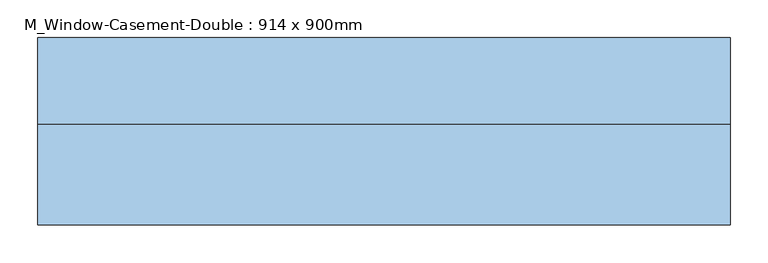
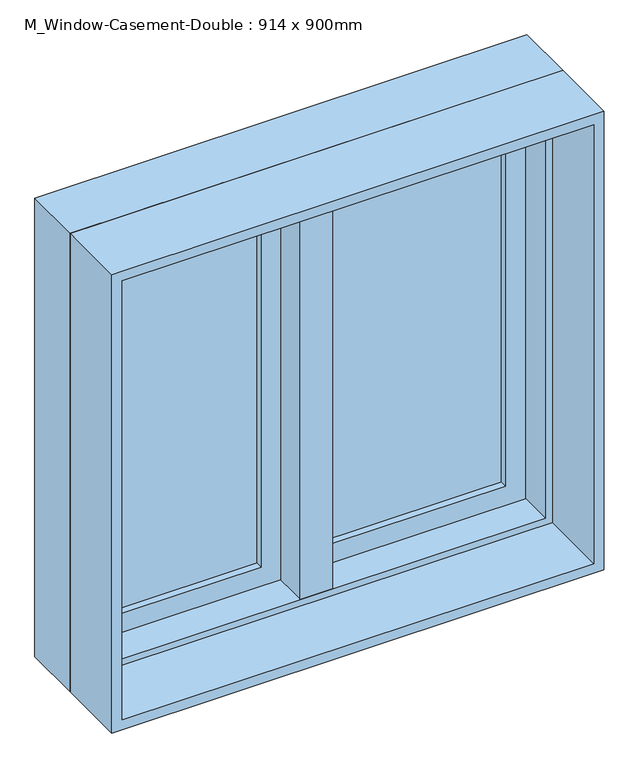
"""IFC4 building model written with IfcOpenShell, lengths in millimetres: window geometry, M_Window-Casement-Double : 914 x 900mm."""

from ifc_helpers import new_model, si_unit, frame, origin, place, context, project, spatial, polyline, outline, extrude, faceted_brep, source, transform, mapped, element, save


def m_window_casement_double_914_x_900mm_7ae2d64b(model_context):
    return source(origin(), model_context, "Body", "SolidModel", [
        faceted_brep([(425.45, 82.55, 1768.25), (425.45, 19.05, 1768.25), (-425.45, 19.05, 1768.25), (-425.45, 82.55, 1768.25), (444.5, 133.35, 1787.3), (444.5, 82.55, 1787.3), (-444.5, 82.55, 1787.3), (-444.5, 133.35, 1787.3), (457.2, 19.05, 1800.0), (457.2, 133.35, 1800.0), (-457.2, 133.35, 1800.0), (-457.2, 19.05, 1800.0), (-425.45, 19.05, 931.75), (-425.45, 82.55, 931.75), (-444.5, 82.55, 912.7), (-444.5, 133.35, 912.7), (-457.2, 133.35, 900.0), (-457.2, 19.05, 900.0), (425.45, 19.05, 931.75), (425.45, 82.55, 931.75), (444.5, 82.55, 912.7), (444.5, 133.35, 912.7), (457.2, 133.35, 900.0), (457.2, 19.05, 900.0)], [[[0, 1, 2, 3]], [[4, 5, 6, 7]], [[8, 9, 10, 11]], [[3, 2, 12, 13]], [[7, 6, 14, 15]], [[11, 10, 16, 17]], [[13, 12, 18, 19]], [[15, 14, 20, 21]], [[17, 16, 22, 23]], [[11, 17, 23, 8], [1, 18, 12, 2]], [[19, 18, 1, 0]], [[5, 20, 14, 6], [3, 13, 19, 0]], [[21, 20, 5, 4]], [[23, 22, 9, 8]], [[9, 22, 16, 10], [7, 15, 21, 4]]]),
        extrude(outline(polyline([(1800.0, -457.2), (900.0, -457.2), (900.0, 457.2), (1800.0, 457.2), (1800.0, -457.2)]), holes=[polyline([(1780.95, 438.15), (919.05, 438.15), (919.05, -438.15), (1780.95, -438.15), (1780.95, 438.15)])]), frame((0.0, -114.3, 0.0), z_axis=(0.0, 1.0, 0.0), x_axis=(0.0, 0.0, 1.0)), (0.0, 0.0, 1.0), 133.35),
        extrude(outline(polyline([(912.7, 444.5), (1787.3, 444.5), (1787.3, 9.525), (912.7, 9.525), (912.7, 444.5)]), holes=[polyline([(969.85, 66.675), (1730.15, 66.675), (1730.15, 387.35), (969.85, 387.35), (969.85, 66.675)])]), frame((0.0, 82.55, 0.0), z_axis=(0.0, 1.0, 0.0), x_axis=(0.0, 0.0, 1.0)), (0.0, 0.0, 1.0), 44.45),
        extrude(outline(polyline([(1787.3, -444.5), (912.7, -444.5), (912.7, -9.525), (1787.3, -9.525), (1787.3, -444.5)]), holes=[polyline([(1730.15, -66.675), (969.85, -66.675), (969.85, -387.35), (1730.15, -387.35), (1730.15, -66.675)])]), frame((0.0, 82.55, 0.0), z_axis=(0.0, 1.0, 0.0), x_axis=(0.0, 0.0, 1.0)), (0.0, 0.0, 1.0), 44.45),
        extrude(outline(polyline([(387.35, 114.3), (387.35, 107.95), (66.675, 107.95), (66.675, 114.3), (387.35, 114.3)])), frame((0.0, 0.0, 969.85), z_axis=(0.0, 0.0, 1.0), x_axis=(1.0, 0.0, 0.0)), (0.0, 0.0, 1.0), 760.3),
        extrude(outline(polyline([(66.675, 95.25), (66.675, 101.6), (387.35, 101.6), (387.35, 95.25), (66.675, 95.25)])), frame((0.0, 0.0, 969.85), z_axis=(0.0, 0.0, 1.0), x_axis=(1.0, 0.0, 0.0)), (0.0, 0.0, 1.0), 760.3),
        extrude(outline(polyline([(-66.675, 114.3), (-66.675, 107.95), (-387.35, 107.95), (-387.35, 114.3), (-66.675, 114.3)])), frame((0.0, 0.0, 969.85), z_axis=(0.0, 0.0, 1.0), x_axis=(1.0, 0.0, 0.0)), (0.0, 0.0, 1.0), 760.3),
        extrude(outline(polyline([(-387.35, 95.25), (-387.35, 101.6), (-66.675, 101.6), (-66.675, 95.25), (-387.35, 95.25)])), frame((0.0, 0.0, 969.85), z_axis=(0.0, 0.0, 1.0), x_axis=(1.0, 0.0, 0.0)), (0.0, 0.0, 1.0), 760.3),
        faceted_brep([(9.525, 133.35, 1787.3), (-9.525, 133.35, 1787.3), (-9.525, 82.55, 1787.3), (9.525, 82.55, 1787.3), (9.525, 133.35, 912.7), (9.525, 82.55, 912.7), (-9.525, 82.55, 912.7), (-9.525, 133.35, 912.7), (-9.525, 82.55, 931.75), (-9.525, 82.55, 1768.25), (-30.1625, 82.55, 931.75), (-30.1625, 82.55, 1768.25), (-30.1625, 19.05, 931.75), (-30.1625, 19.05, 1768.25), (30.1625, 19.05, 931.75), (30.1625, 19.05, 1768.25), (30.1625, 82.55, 931.75), (30.1625, 82.55, 1768.25), (9.525, 82.55, 931.75), (9.525, 82.55, 1768.25)], [[[0, 1, 2, 3]], [[4, 5, 6, 7]], [[1, 0, 4, 7]], [[2, 1, 7, 6, 8, 9]], [[9, 8, 10, 11]], [[11, 10, 12, 13]], [[13, 12, 14, 15]], [[15, 14, 16, 17]], [[17, 16, 18, 19]], [[0, 3, 19, 18, 5, 4]], [[18, 8, 6, 5]], [[9, 19, 3, 2]], [[8, 18, 16, 14, 12, 10]], [[19, 9, 11, 13, 15, 17]]]),
    ])


if __name__ == "__main__":
    model = new_model("IFC4")
    model_context = context("Model", 3, world=origin())
    ifc_project = project(units=[si_unit("LENGTHUNIT", "METRE", prefix="MILLI")], contexts=[model_context])
    site = spatial("IfcSite", under=ifc_project)
    building = spatial("IfcBuilding", under=site)
    placement = place(None, origin())
    m_window_casement_double_914_x_900mm_shape = m_window_casement_double_914_x_900mm_7ae2d64b(model_context)
    element("IfcWindow", 1, ObjectType="M_Window-Casement-Double : 914 x 900mm", at=placement, inside=building, context=model_context, shape_type="MappedRepresentation", body=[
        mapped(m_window_casement_double_914_x_900mm_shape, transform((0.0, 0.0, 0.0), x_axis=(1.0, 0.0, 0.0), y_axis=(0.0, 1.0, 0.0), z_axis=(0.0, 0.0, 1.0))),
    ])
    save(model, "model.ifc")

# Revit data of these elements
# Type "M_Window-Casement-Double : 914 x 900mm"
#   Type Mark = "20"
#   Fire Rating = "0.5h"
#   Assembly Code = "B2020100"
#   Analytic Construction = "Double glazing - domestic"
#   Frame Extension [instance default] = 0' - 0 1/4"
#   Window Inset [instance default] = 0' - 0"
#   Wall Thickness [instance default] = 0' - 5.90551"
#   Interior Wall Closure [instance default] = 0' - 2.15551"
#   Half Width = 1' - 6"
#   Visual Light Transmittance = 0.81
#   Thermal Resistance (R) = 1.8146 (h·ft²·°F)/BTU
#   Solar Heat Gain Coefficient = 0.76
#   Rough Width = 3' - 0.59055"
#   Rough Height = 3' - 0.02362"
#   Height = 2' - 11.43307"
#   Heat Transfer Coefficient (U) = 0.5511 BTU/(h·ft²·°F)
#   Exterior Wall Closure [instance default] = 0' - 1.25197"
#   Extension Jamb [instance default] = 0' - 2.15551"
#   Default Sill Height = 2' - 11.43307"
#   Width = 3' - 0"
#   Muntin Visibility = yes
#   Interior Trim Visibility [instance default] = yes
#   Exterior Trim Visibility [instance default] = yes
#   Extension Jamb Visibility [instance default] = yes
#   Interior Trim Material = Wood - Stained
#   Muntin Pattern = M_Muntin Pattern_2x2 : M_Muntin Pattern_2x2
#   Interior Trim = M_Trim-Window-Interior-Flat : Picture Frame
#   Interior Frame Material = Wood - Stained
#   Glass Panel Material = Glass
#   Exterior Trim Material = Clad - White
#   Exterior Trim = M_Trim-Window-Exterior-Flat : with Sill
#   Exterior Frame Material = Clad - White
#   Wall Closure = (empty or 0)
# Element 1 (IfcWindow, "M_Window-Casement-Double : 914 x 900mm")
#   Wall Thickness = 0' - 9"
#   Extension Jamb = 0' - 5 1/4"
#   Materials on its faces: "Wood - Stained", "Glass", "Clad - White"
# Materials
#   "Wood - Stained": class "Wood", colour RGB 224 178 126, transparency 0, Cost = 0
#   "Glass": class "Glass", colour RGB 0 128 192, transparency 0.75, Description = "Soda Lime Glass", Cost = 0
#   "Clad - White": class "Wood", colour RGB 242 242 238, transparency 0, Cost = 0
